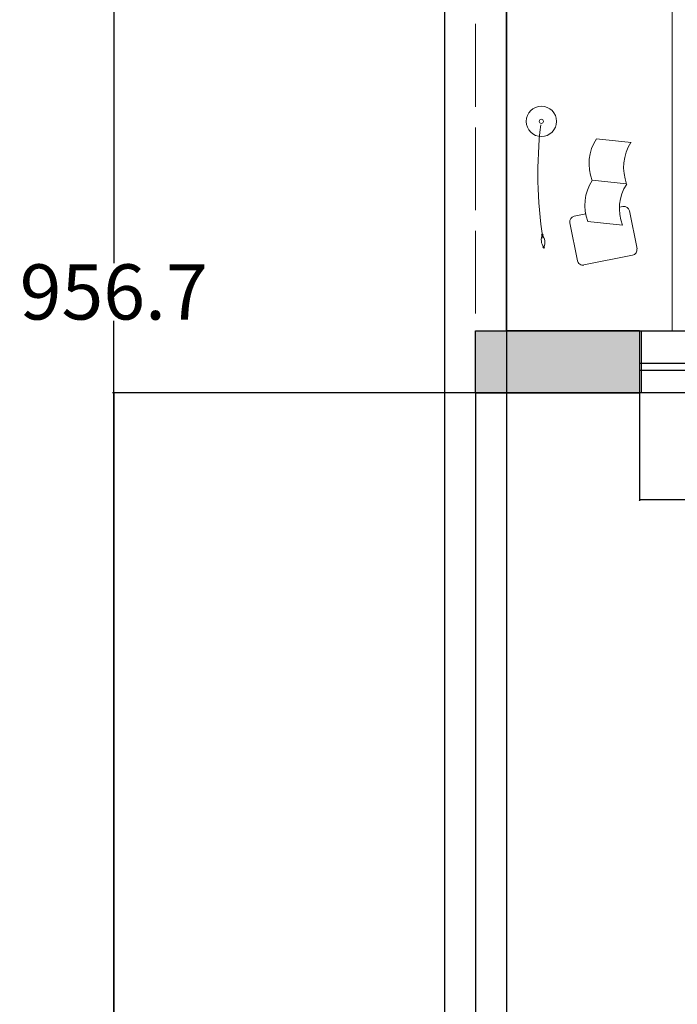
# Model space of a CAD drawing. Units: inches. Extents: x -48 to 50072, y 0 to 21068.
# Tile 59 of 75: x 697 to 793, y 660 to 803. Entities that reach past the tile are written whole.
import ezdxf

# ---------------------------------------------------------------- set-up
doc = ezdxf.new("R2010")
doc.units = ezdxf.units.IN
doc.header["$MEASUREMENT"] = 0
doc.linetypes.add('ACAD_ISO02W100', pattern=[15, 12, -3])
for name, color, linetype, lineweight in [('A-ANNO-DIMS', 2, 'Continuous', 18), ('A-COLS', 1, 'Continuous', 35), ('A-DOOR', 4, 'Continuous', 18), ('A-FLOR-CASE', 9, 'Continuous', 18), ('A-WALL', 7, 'Continuous', 35), ('C-PROP', 7, 'Continuous', 25), ('C-PROP-REF', 32, 'ACAD_ISO02W100', 13), ('FURNITURE', 44, 'Continuous', 18)]:
    doc.layers.add(name, color=color, linetype=linetype, lineweight=lineweight)
doc.layers.add('Layer3', color=176, linetype='Continuous')
doc.styles.get("Standard").update_dxf_attribs({"font": 'arial.ttf'})
doc.dimstyles.get("Standard").update_dxf_attribs({"dimtxt": 8, "dimasz": 0.18, "dimexe": 0.18, "dimexo": 0.0625, "dimgap": 0.09, "dimtad": 0, "dimtih": 1, "dimtoh": 1, "dimdec": 1, "dimzin": 0, "dimdsep": 46, "dimlunit": 4, "dimtxsty": 'Standard', "dimblk": 'ARCHTICK', "dimcen": 0.09, "dimadec": 0, "dimazin": 0, "dimtfac": 1, "dimtdec": 1, "dimtofl": 0, "dimtmove": 0, "dimatfit": 3, "dimldrblk": 'ARCHTICK', "dimfxl": 1, "dimtolj": 1, "dimtzin": 0, "dimarcsym": 0})

# ---------------------------------------------------------------- blocks, each defined once
blk = doc.blocks.new('bnniku')
at = {"layer": 'Defpoints'}
h = blk.add_hatch(color=256, dxfattribs=at)
h.dxf.hatch_style = 1
h.paths.add_polyline_path([(767.55, 1114.04), (758.55, 1114.04), (758.55, 1090.04), (767.55, 1090.04)])
for p, q in [((758.55, 1114.04), (767.55, 1114.04)), ((758.55, 1090.04), (758.55, 1114.04)), ((767.55, 1114.04), (767.55, 1090.04)), ((767.55, 1090.04), (758.55, 1090.04))]:
    blk.add_line(p, q, dxfattribs=at)
blk = doc.blocks.new('fdsghhhhhhygr')
for p, q in [((41.77, 686.77), (41.77, 677.77)), ((144.77, 677.77), (144.77, 686.77))]:
    blk.add_line(p, q)
at = {"layer": 'Defpoints'}
for p, q in [((91.27, 683.47), (144.77, 683.47)), ((91.27, 683.47), (91.27, 682.47)), ((91.27, 682.47), (144.77, 682.47)), ((41.77, 682.07), (95.27, 682.07)), ((41.77, 681.07), (95.27, 681.07)), ((95.27, 682.07), (95.27, 681.07))]:
    blk.add_line(p, q, dxfattribs=at)
at = {"layer": 'Layer3'}
for p, q in [((41.77, 686.77), (144.77, 686.77)), ((144.77, 677.77), (41.77, 677.77))]:
    blk.add_line(p, q, dxfattribs=at)
blk = doc.blocks.new('DESK-ACCESSORIES')
for p, q in [((10.18, 18.3), (15.19, 17.78)), ((9.56, 12.3), (14.56, 11.78)), ((6.96, 7.08), (8.64, 7.41)), ((13.5, 8.38), (14.02, 8.49)), ((14.96, 7.86), (16.06, 2.37)), ((7.43, 0.64), (6.33, 6.13)), ((13.94, 5.81), (8.93, 6.33)), ((15.43, 1.43), (8.37, 0.02))]:
    blk.add_line(p, q)
for centre, radius, start, end in [((2.2, 20.84), 2.2, 90, 270), ((2.2, 20.84), 2.2, 270, 90), ((63.85, 13.23), 62.16, 173.4513, 188.6305), ((2.2, 20.84), 0.3, 90, 270), ((2.2, 20.84), 0.3, 270, 90), ((15.87, 14.66), 6.76, 147.37, 200.7442), ((20.88, 14.14), 6.76, 147.37, 200.7442), ((15.03, 8.7), 6.54, 146.9045, 201.2097), ((20.04, 8.18), 6.54, 146.9045, 201.2097), ((14.18, 7.7), 0.8, 11.3025, 101.3025), ((7.12, 6.29), 0.8, 101.3025, 191.3025), ((4, 3.71), 1.82, 157.356, 216.9378), ((2.33, 4.39), 0.12, 90, 270), ((0.87, 3.31), 1.82, 337.356, 36.9378), ((2.33, 4.39), 0.12, 270, 90), ((2.54, 2.6), 0.12, 90, 270), ((2.54, 2.6), 0.12, 270, 90), ((15.27, 2.21), 0.8, 281.3025, 11.3025), ((8.21, 0.8), 0.8, 191.3025, 281.3025)]:
    blk.add_arc(centre, radius, start, end)
blk = doc.blocks.new('_ArchTick')
at = {"color": 0, "linetype": 'ByBlock', "const_width": 0.15}
blk.add_lwpolyline([(-0.5, -0.5), (0.5, 0.5)], dxfattribs=at)
blk = doc.blocks.new('*D60')
at = {"layer": 'A-ANNO-DIMS', "color": 0, "lineweight": -2, "transparency": 16777216}
for p, q in [((787.01, 748.4), (787.01, 732.83)), ((890.01, 748.4), (890.01, 732.83)), ((787.01, 733.01), (890.01, 733.01)), ((890.01, 733.01), (890.19, 733.01))]:
    blk.add_line(p, q, dxfattribs=at)
at = {"layer": 'Defpoints', "color": 0, "transparency": 16777216}
for p in [(787.01, 748.46), (890.01, 748.46), (890.01, 733.01)]:
    blk.add_point(p, dxfattribs=at)
at = {"layer": 'A-ANNO-DIMS', "color": 0, "lineweight": -2, "transparency": 16777216, "xscale": 0.18, "yscale": 0.18, "zscale": 0.18, "rotation": 180}
blk.add_blockref('_ArchTick', (787.01, 733.01), dxfattribs=at)
at = {"layer": 'A-ANNO-DIMS', "color": 0, "lineweight": -2, "transparency": 16777216, "xscale": 0.18, "yscale": 0.18, "zscale": 0.18}
blk.add_blockref('_ArchTick', (890.01, 733.01), dxfattribs=at)
at = {"layer": 'A-ANNO-DIMS', "color": 0, "transparency": 16777216, "insert": (960.35, 733.01), "char_height": 8, "attachment_point": 5}
blk.add_mtext('\\A1;SLIDING DOOR A 103 TYP.', dxfattribs=at)
blk = doc.blocks.new('*D130')
at = {"layer": 'A-ANNO-DIMS', "color": 0, "lineweight": -2, "transparency": 16777216}
for p, q in [((758.7, 1241.46), (710.63, 1241.46)), ((710.81, 1241.46), (710.81, 767.29)), ((710.81, 284.76), (710.81, 758.94)), ((758.7, 284.76), (710.63, 284.76))]:
    blk.add_line(p, q, dxfattribs=at)
at = {"layer": 'Defpoints', "color": 0, "transparency": 16777216}
for p in [(710.81, 1241.46), (758.76, 1241.46), (758.76, 284.76)]:
    blk.add_point(p, dxfattribs=at)
at = {"layer": 'A-ANNO-DIMS', "color": 0, "lineweight": -2, "transparency": 16777216, "xscale": 0.18, "yscale": 0.18, "zscale": 0.18}
for p, rotation in [((710.81, 1241.46), 90), ((710.81, 284.76), 270)]:
    blk.add_blockref('_ArchTick', p, dxfattribs=dict(at, rotation=rotation))
at = {"layer": 'A-ANNO-DIMS', "color": 0, "transparency": 16777216, "insert": (710.81, 763.11), "char_height": 8, "attachment_point": 5}
blk.add_mtext('\\A1;956.7', dxfattribs=at)
blk = doc.blocks.new('*D135')
at = {"layer": 'A-ANNO-DIMS', "color": 0, "lineweight": -2, "transparency": 16777216}
for p, q in [((763.26, 748.4), (763.26, 236.63)), ((909.26, 748.4), (909.26, 236.63)), ((763.26, 236.81), (827.71, 236.81)), ((909.26, 236.81), (844.81, 236.81))]:
    blk.add_line(p, q, dxfattribs=at)
at = {"layer": 'Defpoints', "color": 0, "transparency": 16777216}
for p in [(763.26, 748.46), (909.26, 748.46), (909.26, 236.81)]:
    blk.add_point(p, dxfattribs=at)
at = {"layer": 'A-ANNO-DIMS', "color": 0, "lineweight": -2, "transparency": 16777216, "xscale": 0.18, "yscale": 0.18, "zscale": 0.18, "rotation": 180}
blk.add_blockref('_ArchTick', (763.26, 236.81), dxfattribs=at)
at = {"layer": 'A-ANNO-DIMS', "color": 0, "lineweight": -2, "transparency": 16777216, "xscale": 0.18, "yscale": 0.18, "zscale": 0.18}
blk.add_blockref('_ArchTick', (909.26, 236.81), dxfattribs=at)
at = {"layer": 'A-ANNO-DIMS', "color": 0, "transparency": 16777216, "insert": (836.26, 236.81), "char_height": 8, "attachment_point": 5}
blk.add_mtext('\\A1;146', dxfattribs=at)
blk = doc.blocks.new('*D145')
at = {"layer": 'A-ANNO-DIMS', "color": 0, "lineweight": -2, "transparency": 16777216}
for p, q in [((961.2, 748.46), (710.63, 748.46)), ((710.81, 748.46), (710.81, 658.14)), ((710.81, 559.46), (710.81, 649.79)), ((961.2, 559.46), (710.63, 559.46))]:
    blk.add_line(p, q, dxfattribs=at)
at = {"layer": 'Defpoints', "color": 0, "transparency": 16777216}
for p in [(710.81, 748.46), (961.26, 748.46), (961.26, 559.46)]:
    blk.add_point(p, dxfattribs=at)
at = {"layer": 'A-ANNO-DIMS', "color": 0, "lineweight": -2, "transparency": 16777216, "xscale": 0.18, "yscale": 0.18, "zscale": 0.18}
for p, rotation in [((710.81, 748.46), 90), ((710.81, 559.46), 270)]:
    blk.add_blockref('_ArchTick', p, dxfattribs=dict(at, rotation=rotation))
at = {"layer": 'A-ANNO-DIMS', "color": 0, "transparency": 16777216, "insert": (710.81, 653.96), "char_height": 8, "attachment_point": 5}
blk.add_mtext('\\A1;189', dxfattribs=at)

msp = doc.modelspace()

# ---------------------------------------------------------------- linework, layer by layer
at = {"layer": 'A-FLOR-CASE'}
msp.add_line((791.761, 757.464), (791.761, 874.822), dxfattribs=at)
at = {"layer": 'A-WALL'}
for p, q in [((767.761, 757.464), (767.761, 841.464)), ((787.01, 757.464), (767.761, 757.464)), ((787.01, 748.464), (763.261, 748.464))]:
    msp.add_line(p, q, dxfattribs=at)
at = {"layer": 'C-PROP'}
for p, q in [((758.761, 1241.464), (758.761, 284.764)), ((767.761, 931.464), (767.761, 293.764))]:
    msp.add_line(p, q, dxfattribs=at)
at = {"layer": 'C-PROP-REF'}
msp.add_line((763.261, 1236.964), (763.261, 284.764), dxfattribs=at)

# ---------------------------------------------------------------- block references
at = {"layer": 'A-COLS', "rotation": 90}
msp.add_blockref('bnniku', (1877.298, -10.088), dxfattribs=at)
at = {"layer": 'A-DOOR'}
msp.add_blockref('fdsghhhhhhygr', (745.244, 70.689), dxfattribs=at)
at = {"layer": 'FURNITURE'}
msp.add_blockref('DESK-ACCESSORIES', (770.607, 767), dxfattribs=at)

# ---------------------------------------------------------------- dimensions: what is measured, and where the dimension line sits
at = {"layer": 'A-ANNO-DIMS'}
for base, p1, p2, override, picture, middle in [((710.811, 1241.464), (758.761, 284.764), (758.761, 1241.464), {"dimdec": 1, "dimlfac": 1, "dimrnd": 0, "dimzin": 0, "dimdsep": 46, "dimlunit": 2}, '*D130', (710.811, 763.114)), ((710.811, 748.464), (961.261, 559.464), (961.261, 748.464), {"dimdec": 0, "dimlfac": 1, "dimrnd": 0, "dimzin": 0, "dimdsep": 46, "dimlunit": 2}, '*D145', (710.811, 653.964))]:
    dim = msp.add_linear_dim(base=base, p1=p1, p2=p2, angle=90, dimstyle='Standard', override=override, dxfattribs=at)
    dim.commit()
    dim.dimension.update_dxf_attribs({"geometry": picture, "text_midpoint": middle})
dim = msp.add_linear_dim(base=(890.012, 733.014), p1=(787.01, 748.464), p2=(890.012, 748.464), text='SLIDING DOOR A <> TYP.', dimstyle='Standard', override={"dimdec": 0, "dimlfac": 1, "dimrnd": 0, "dimzin": 0, "dimdsep": 46, "dimlunit": 2}, dxfattribs=at)
dim.commit()
dim.dimension.update_dxf_attribs({"geometry": '*D60', "text_midpoint": (960.347, 733.014)})
dim = msp.add_linear_dim(base=(909.261, 236.814), p1=(763.261, 748.464), p2=(909.261, 748.464), dimstyle='Standard', override={"dimdec": 0, "dimlfac": 1, "dimrnd": 0, "dimzin": 0, "dimdsep": 46, "dimlunit": 2}, dxfattribs=at)
dim.commit()
dim.dimension.update_dxf_attribs({"geometry": '*D135', "text_midpoint": (836.261, 236.814)})

doc.saveas('drawing.dxf')
